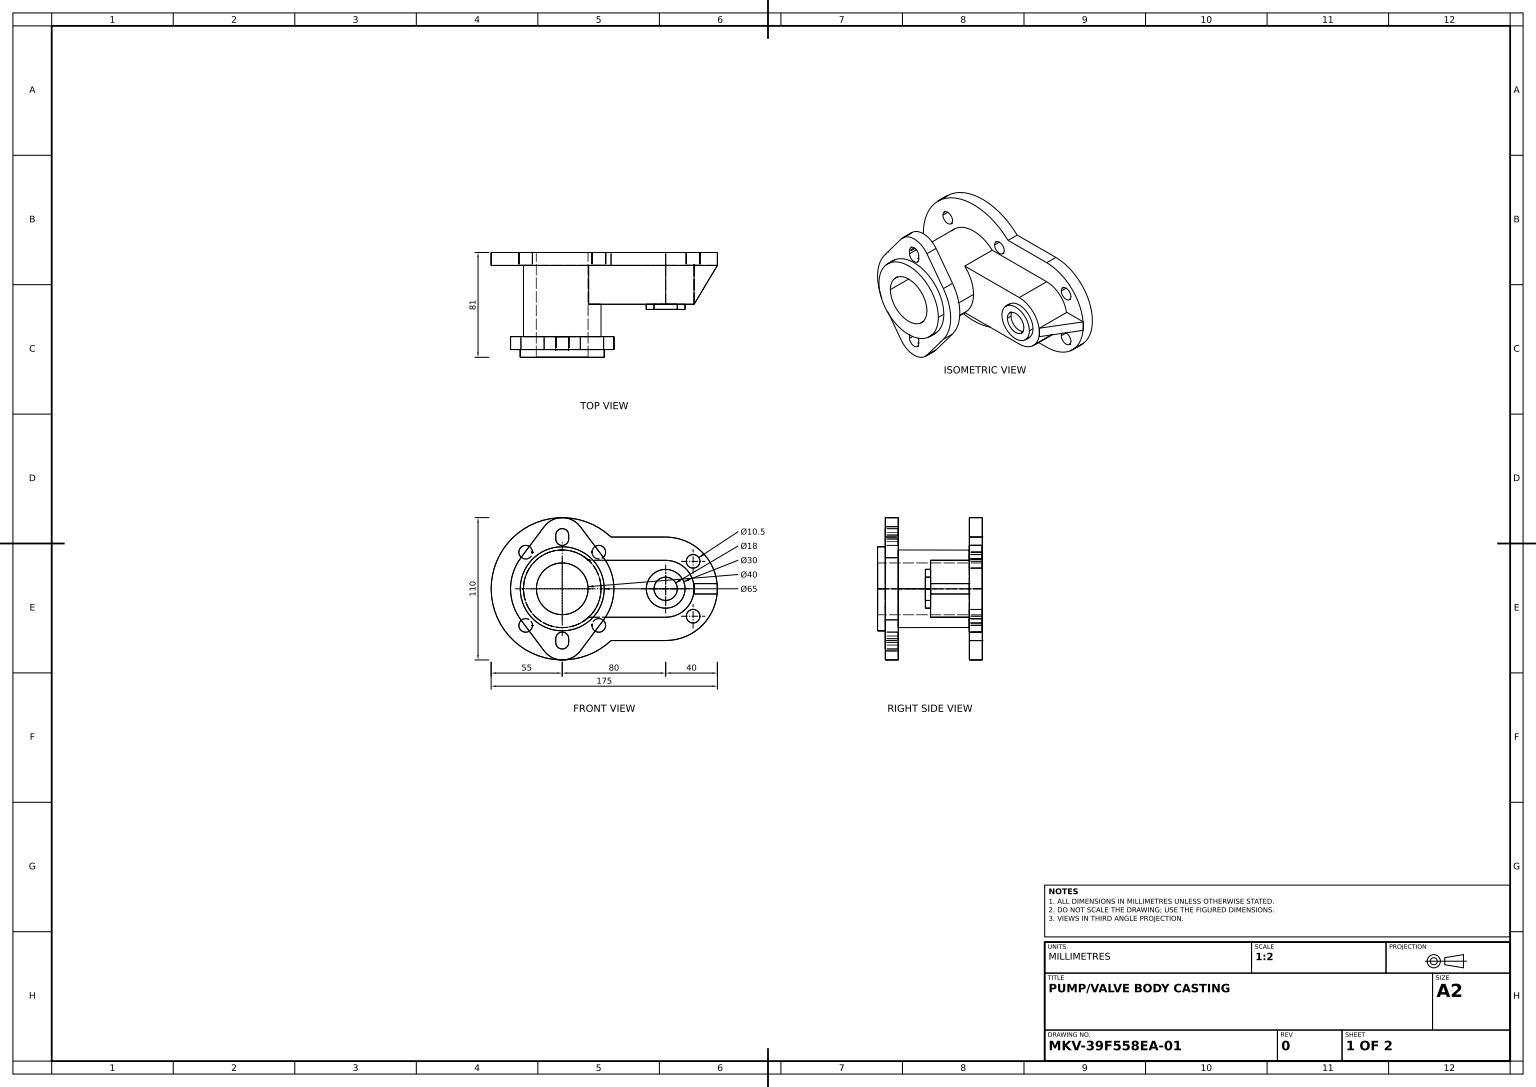
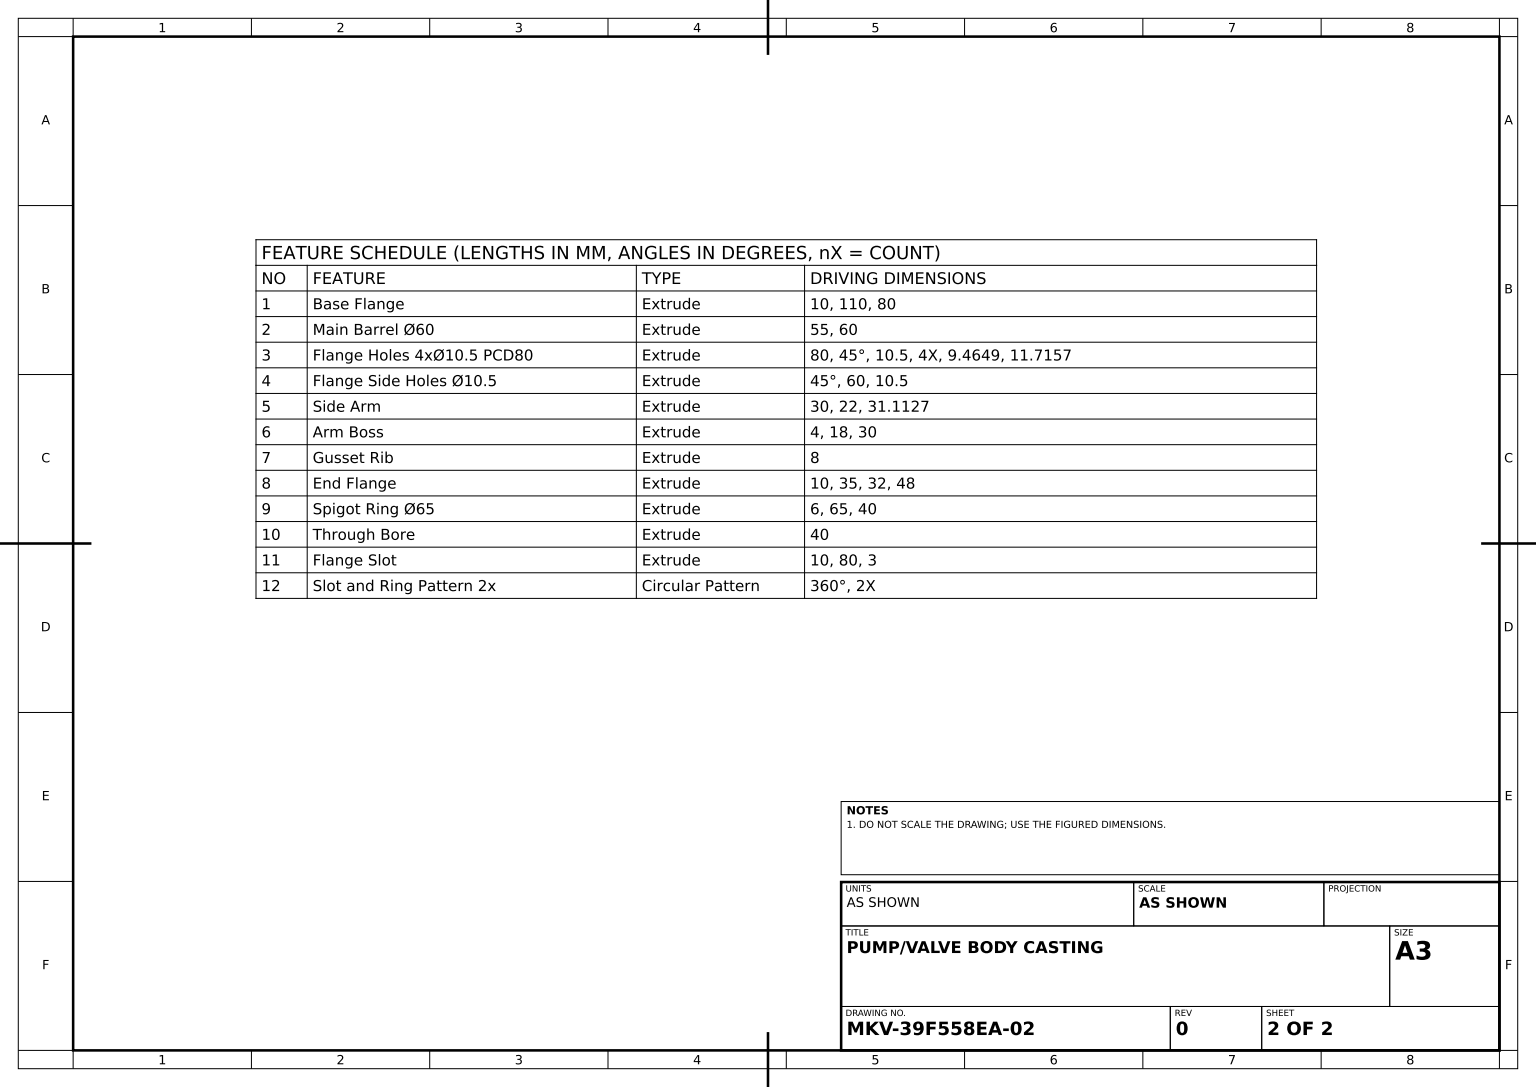
from build123d import *

# Parameters (mm, degrees)
BASE_FLANGE_DEPTH                = 10
MAIN_BARREL_SKETCH_R             = 30
MAIN_BARREL_60_DEPTH             = 55
FLANGE_HOLES_SKETCH_R            = 5.25
FLANGE_HOLES_4X_10_5_PCD80_DEPTH = 144.003496461
FLANGE_SIDE_HOLES_SKETCH_R       = 5.25
FLANGE_SIDE_HOLES_10_5_DEPTH     = 144.003496461
SIDE_ARM_DEPTH                   = 30
ARM_BOSS_SKETCH_R                = 15
ARM_BOSS_SKETCH_R_2              = 9
ARM_BOSS_DEPTH                   = 4
GUSSET_RIB_DEPTH                 = 4
END_FLANGE_DEPTH                 = 10
SPIGOT_RING_SKETCH_R             = 32.5
SPIGOT_RING_SKETCH_R_2           = 20
SPIGOT_RING_65_DEPTH             = 6
THROUGH_BORE_SKETCH_R            = 20
THROUGH_BORE_DEPTH               = 152.822264507
FLANGE_SLOT_DEPTH                = 10
SLOT_AND_RING_PATTERN_2X_COUNT   = 2


with BuildPart() as part:
    # Base Flange Sketch → Base Flange (new body)
    with BuildSketch(Plane.XY):
        with BuildLine():
            Line((80, 40), (37.749172176, 40))
            ThreePointArc((37.749172176, 40), (-55, 0), (37.749172176, -40))
            Line((37.749172176, -40), (80, -40))
            ThreePointArc((80, -40), (120, 0), (80, 40))
        make_face()
    extrude(amount=BASE_FLANGE_DEPTH)

    # Main Barrel Sketch → Main Barrel Ø60 (add)
    with BuildSketch(Plane.XY.offset(10)):
        Circle(MAIN_BARREL_SKETCH_R)
    extrude(amount=MAIN_BARREL_60_DEPTH)

    # Flange Holes Sketch → Flange Holes 4xØ10.5 PCD80 (cut, through all)
    with BuildSketch(Plane.XY.offset(10)):
        with Locations((28.284271247, 28.284271247)):
            Circle(FLANGE_HOLES_SKETCH_R)
        with Locations((28.284271247, -28.284271247)):
            Circle(FLANGE_HOLES_SKETCH_R)
        with Locations((-28.284271247, -28.284271247)):
            Circle(FLANGE_HOLES_SKETCH_R)
        with Locations((-28.284271247, 28.284271247)):
            Circle(FLANGE_HOLES_SKETCH_R)
    extrude(amount=-FLANGE_HOLES_4X_10_5_PCD80_DEPTH, mode=Mode.SUBTRACT)

    # Flange Side Holes Sketch → Flange Side Holes Ø10.5 (cut, through all)
    with BuildSketch(Plane.XY.offset(10)):
        with Locations((101.213203436, 21.213203436)):
            Circle(FLANGE_SIDE_HOLES_SKETCH_R)
        with Locations((101.213203436, -21.213203436)):
            Circle(FLANGE_SIDE_HOLES_SKETCH_R)
    extrude(amount=-FLANGE_SIDE_HOLES_10_5_DEPTH, mode=Mode.SUBTRACT)

    # Side Arm Sketch → Side Arm (add)
    with BuildSketch(Plane.XY.offset(10)):
        with BuildLine():
            Line((80, 22), (20.396078054, 22))
            ThreePointArc((20.396078054, 22), (29.508776427, 0), (20.396078054, -22))
            Line((20.396078054, -22), (80, -22))
            ThreePointArc((80, -22), (102, 0), (80, 22))
        make_face()
    extrude(amount=SIDE_ARM_DEPTH)

    # Arm Boss Sketch → Arm Boss (add)
    with BuildSketch(Plane.XY.offset(40)):
        with Locations((80, 0)):
            Circle(ARM_BOSS_SKETCH_R)
        with Locations((80, 0)):
            Circle(ARM_BOSS_SKETCH_R_2, mode=Mode.SUBTRACT)
    extrude(amount=ARM_BOSS_DEPTH)

    # End Flange Sketch → End Flange (add)
    with BuildSketch(Plane.XY.offset(65)):
        with BuildLine():
            Line((14, 48), (32, 24))
            ThreePointArc((32, 24), (40, 0), (32, -24))
            Line((32, -24), (14, -48))
            ThreePointArc((14, -48), (0, -55), (-14, -48))
            Line((-14, -48), (-32, -24))
            ThreePointArc((-32, -24), (-40, 0), (-32, 24))
            Line((-32, 24), (-14, 48))
            ThreePointArc((-14, 48), (0, 55), (14, 48))
        make_face()
    extrude(amount=END_FLANGE_DEPTH)

    # Spigot Ring Sketch → Spigot Ring Ø65 (add)
    with BuildSketch(Plane.XY.offset(75)):
        Circle(SPIGOT_RING_SKETCH_R)
        Circle(SPIGOT_RING_SKETCH_R_2, mode=Mode.SUBTRACT)
    extrude(amount=SPIGOT_RING_65_DEPTH)

    # Through Bore Sketch → Through Bore (cut, through all)
    with BuildSketch(Plane.XY.offset(75)):
        Circle(THROUGH_BORE_SKETCH_R)
    extrude(amount=-THROUGH_BORE_DEPTH, mode=Mode.SUBTRACT)

    # Flange Slot Sketch → Flange Slot (cut)
    with BuildSketch(Plane.XY.offset(75)):
        with BuildLine():
            Line((-5, 38.5), (-5, 41.5))
            ThreePointArc((-5, 41.5), (0, 46.5), (5, 41.5))
            Line((5, 41.5), (5, 38.5))
            ThreePointArc((5, 38.5), (0, 33.5), (-5, 38.5))
        make_face()
    flange_slot = extrude(amount=-FLANGE_SLOT_DEPTH, mode=Mode.SUBTRACT)

    # Slot and Ring Pattern 2x: Flange Slot ×2 about axis
    slot_and_ring_pattern_2x_axis = Axis((0, 0, 0), (0, 0, 1))
    for i in range(1, SLOT_AND_RING_PATTERN_2X_COUNT):
        add(flange_slot.rotate(slot_and_ring_pattern_2x_axis, i * 360 / SLOT_AND_RING_PATTERN_2X_COUNT), mode=Mode.SUBTRACT)


with BuildPart() as body_2:
    # Gusset Rib Sketch → Gusset Rib (new, symmetric)
    with BuildSketch(Plane(origin=(0, 0, 0), x_dir=(1, 0, 0), z_dir=(0, 1, 0))):
        Polygon((102, -40), (120, -10), (102, -10), align=None)
    extrude(amount=GUSSET_RIB_DEPTH, both=True)


solid = Compound([part.part, body_2.part])
